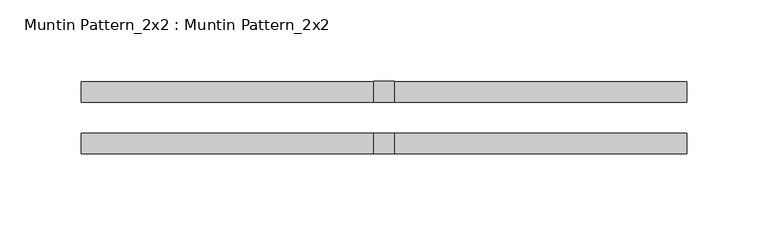
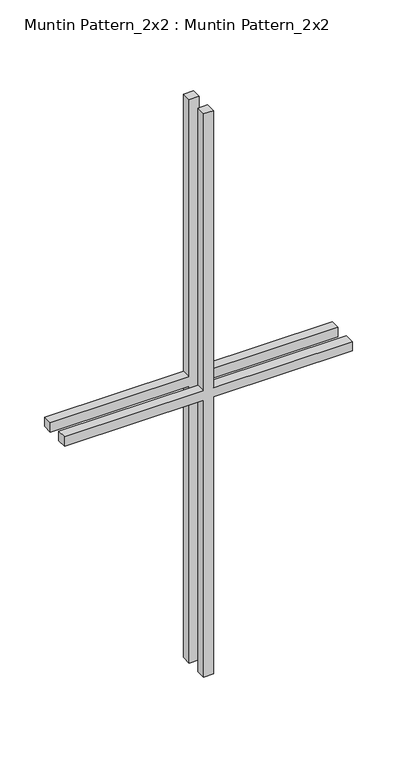
"""IFC4 building model written with IfcOpenShell, lengths in millimetres: proxy geometry, Muntin Pattern_2x2 : Muntin Pattern_2x2."""

from ifc_helpers import new_model, si_unit, frame, origin, place, context, project, spatial, polyline, outline, extrude, source, transform, mapped, element, save


def muntin_pattern_2x2_muntin_pattern_2x2_5e7f5336(model_context):
    return source(origin(), model_context, "Body", "SweptSolid", [
        extrude(outline(polyline([(390.525, -6.35), (390.525, -185.7375), (377.825, -185.7375), (377.825, -6.35), (0.0, -6.35), (0.0, 6.35), (377.825, 6.35), (377.825, 185.7375), (390.525, 185.7375), (390.525, 6.35), (768.35, 6.35), (768.35, -6.35), (390.525, -6.35)])), frame((0.0, 9.525, 0.0), z_axis=(0.0, 1.0, 0.0), x_axis=(0.0, 0.0, 1.0)), (0.0, 0.0, 1.0), 12.7),
        extrude(outline(polyline([(390.525, -6.35), (390.525, -185.7375), (377.825, -185.7375), (377.825, -6.35), (0.0, -6.35), (0.0, 6.35), (377.825, 6.35), (377.825, 185.7375), (390.525, 185.7375), (390.525, 6.35), (768.35, 6.35), (768.35, -6.35), (390.525, -6.35)])), frame((0.0, -22.225, 0.0), z_axis=(0.0, 1.0, 0.0), x_axis=(0.0, 0.0, 1.0)), (0.0, 0.0, 1.0), 12.7),
    ])


if __name__ == "__main__":
    model = new_model("IFC4")
    model_context = context("Model", 3, world=origin())
    ifc_project = project(units=[si_unit("LENGTHUNIT", "METRE", prefix="MILLI")], contexts=[model_context])
    site = spatial("IfcSite", under=ifc_project)
    building = spatial("IfcBuilding", under=site)
    placement = place(None, origin())
    muntin_pattern_2x2_muntin_pattern_2x2_shape = muntin_pattern_2x2_muntin_pattern_2x2_5e7f5336(model_context)
    element("IfcBuildingElementProxy", 1, Name="Muntin Pattern_2x2 : Muntin Pattern_2x2", ObjectType="Muntin Pattern_2x2 : Muntin Pattern_2x2", at=placement, inside=building, context=model_context, shape_type="MappedRepresentation", body=[
        mapped(muntin_pattern_2x2_muntin_pattern_2x2_shape, transform((0.0, 0.0, 0.0), x_axis=(1.0, 0.0, 0.0), y_axis=(0.0, 1.0, 0.0), z_axis=(0.0, 0.0, 1.0))),
    ])
    save(model, "model.ifc")

# Revit data of these elements
# Type "Muntin Pattern_2x2 : Muntin Pattern_2x2"
#   Width [instance default] = 4' - 0"
#   Thickness = 0' - 0 1/2"
#   Height [instance default] = 4' - 0"
#   Distance = 0' - 0 3/4"
#   Interior Material [instance default] = none
#   Exterior Material [instance default] = none
#   Default Elevation = 0
# Element 1 (IfcBuildingElementProxy, "Muntin Pattern_2x2 : Muntin Pattern_2x2")
#   Width = 1' - 2 5/8"
#   Height = 2' - 6 1/4"
#   Interior Material = Wood - Stained
#   Exterior Material = Clad - White
#   Materials on its faces: "Clad - White", "Wood - Stained"
# Materials
#   "Clad - White": class "Wood", colour RGB 242 242 238, transparency 0, Cost = 0
#   "Wood - Stained": class "Wood", colour RGB 227 170 128, transparency 0, Cost = 0
